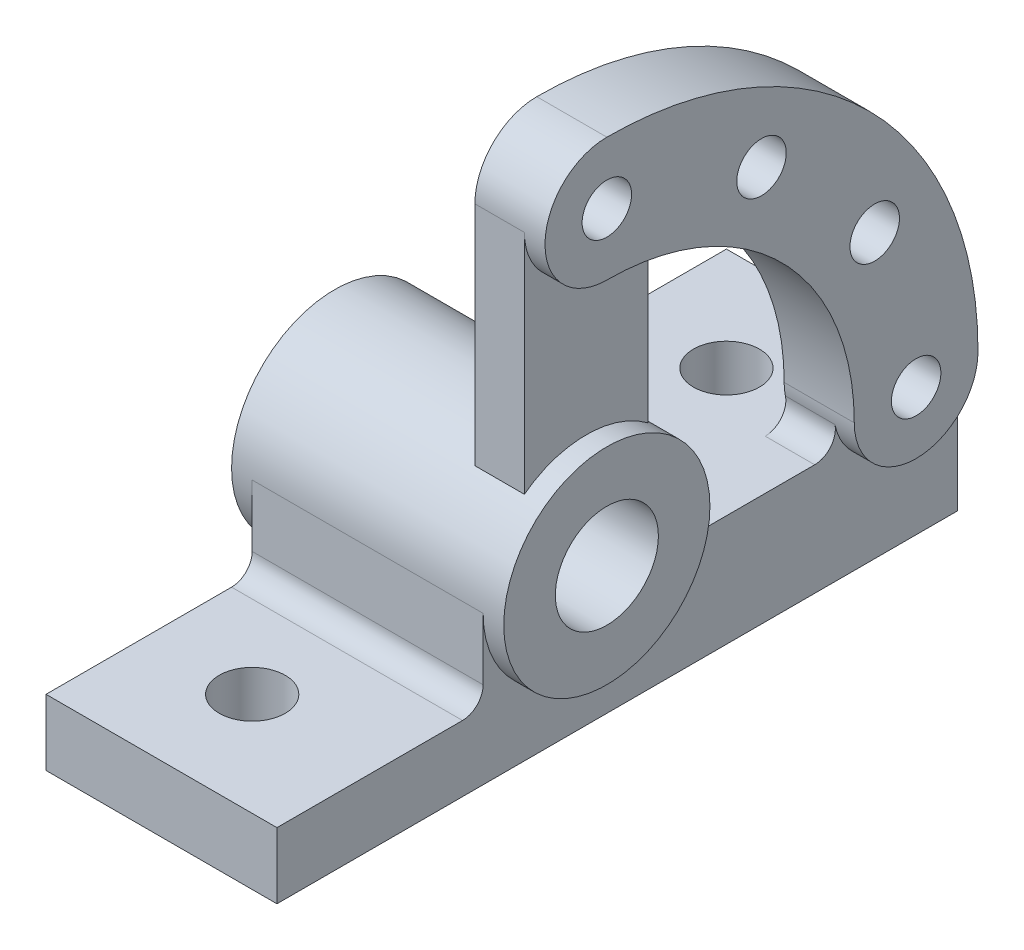
ISO-10303-21;
HEADER;
FILE_DESCRIPTION(('STEP AP214'),'2;1');
FILE_NAME('part.step','',(''),(''),'','','');
FILE_SCHEMA(('AUTOMOTIVE_DESIGN { 1 0 10303 214 1 1 1 1 }'));
ENDSEC;
DATA;
#1=APPLICATION_CONTEXT('core data for automotive mechanical design processes');
#2=APPLICATION_PROTOCOL_DEFINITION('international standard','automotive_design',2000,#1);
#3=PRODUCT_CONTEXT('',#1,'mechanical');
#4=PRODUCT('Part','Part','',(#3));
#5=PRODUCT_RELATED_PRODUCT_CATEGORY('part','',(#4));
#6=PRODUCT_DEFINITION_FORMATION('','',#4);
#7=PRODUCT_DEFINITION_CONTEXT('part definition',#1,'design');
#8=PRODUCT_DEFINITION('design','',#6,#7);
#9=PRODUCT_DEFINITION_SHAPE('','',#8);
#10=(LENGTH_UNIT() NAMED_UNIT(*) SI_UNIT(.MILLI.,.METRE.));
#11=(NAMED_UNIT(*) PLANE_ANGLE_UNIT() SI_UNIT($,.RADIAN.));
#12=(NAMED_UNIT(*) SI_UNIT($,.STERADIAN.) SOLID_ANGLE_UNIT());
#13=UNCERTAINTY_MEASURE_WITH_UNIT(LENGTH_MEASURE(1.E-05),#10,'distance_accuracy_value','');
#14=(GEOMETRIC_REPRESENTATION_CONTEXT(3) GLOBAL_UNCERTAINTY_ASSIGNED_CONTEXT((#13)) GLOBAL_UNIT_ASSIGNED_CONTEXT((#10,
#11,#12)) REPRESENTATION_CONTEXT('',''));
#15=CARTESIAN_POINT('',(0.,0.,0.));
#16=DIRECTION('',(0.,0.,1.));
#17=DIRECTION('',(1.,0.,0.));
#18=AXIS2_PLACEMENT_3D('',#15,#16,#17);
#19=CARTESIAN_POINT('',(16.,0.,0.));
#20=DIRECTION('',(1.,0.,0.));
#21=DIRECTION('',(0.,0.,-1.));
#22=AXIS2_PLACEMENT_3D('',#19,#20,#21);
#23=PLANE('',#22);
#24=CARTESIAN_POINT('',(16.,0.,-75.));
#25=DIRECTION('',(1.,0.,0.));
#26=DIRECTION('',(0.,0.,-1.));
#27=AXIS2_PLACEMENT_3D('',#24,#25,#26);
#28=CIRCLE('',#27,6.);
#29=CARTESIAN_POINT('',(16.,0.,-81.));
#30=VERTEX_POINT('',#29);
#31=EDGE_CURVE('E209',#30,#30,#28,.F.);
#32=ORIENTED_EDGE('',*,*,#31,.F.);
#33=EDGE_LOOP('',(#32));
#34=FACE_BOUND('',#33,.T.);
#35=CARTESIAN_POINT('',(16.,75.,2.61861100413235E-13));
#36=DIRECTION('',(1.,0.,0.));
#37=DIRECTION('',(0.,0.,-1.));
#38=AXIS2_PLACEMENT_3D('',#35,#36,#37);
#39=CIRCLE('',#38,6.);
#40=CARTESIAN_POINT('',(16.,75.,-5.99999999999974));
#41=VERTEX_POINT('',#40);
#42=EDGE_CURVE('E393',#41,#41,#39,.F.);
#43=ORIENTED_EDGE('',*,*,#42,.F.);
#44=EDGE_LOOP('',(#43));
#45=FACE_BOUND('',#44,.T.);
#46=CARTESIAN_POINT('',(16.,64.951905283833,-37.4999999999998));
#47=DIRECTION('',(1.,0.,0.));
#48=DIRECTION('',(0.,0.,-1.));
#49=AXIS2_PLACEMENT_3D('',#46,#47,#48);
#50=CIRCLE('',#49,6.);
#51=CARTESIAN_POINT('',(16.,64.951905283833,-43.4999999999999));
#52=VERTEX_POINT('',#51);
#53=EDGE_CURVE('E397',#52,#52,#50,.F.);
#54=ORIENTED_EDGE('',*,*,#53,.F.);
#55=EDGE_LOOP('',(#54));
#56=FACE_BOUND('',#55,.T.);
#57=CARTESIAN_POINT('',(16.,37.5000000000001,-64.9519052838328));
#58=DIRECTION('',(1.,0.,0.));
#59=DIRECTION('',(0.,0.,-1.));
#60=AXIS2_PLACEMENT_3D('',#57,#58,#59);
#61=CIRCLE('',#60,6.);
#62=CARTESIAN_POINT('',(16.,37.5000000000001,-70.9519052838329));
#63=VERTEX_POINT('',#62);
#64=EDGE_CURVE('E388',#63,#63,#61,.F.);
#65=ORIENTED_EDGE('',*,*,#64,.F.);
#66=EDGE_LOOP('',(#65));
#67=FACE_BOUND('',#66,.T.);
#68=CARTESIAN_POINT('',(16.,0.,0.));
#69=DIRECTION('',(1.,0.,0.));
#70=DIRECTION('',(0.,0.,-1.));
#71=AXIS2_PLACEMENT_3D('',#68,#69,#70);
#72=CIRCLE('',#71,90.);
#73=CARTESIAN_POINT('',(16.,90.,0.));
#74=VERTEX_POINT('',#73);
#75=CARTESIAN_POINT('',(16.,0.,-90.));
#76=VERTEX_POINT('',#75);
#77=EDGE_CURVE('E198',#74,#76,#72,.F.);
#78=ORIENTED_EDGE('',*,*,#77,.T.);
#79=DIRECTION('',(0.,1.,0.));
#80=VECTOR('',#79,1.);
#81=CARTESIAN_POINT('',(16.,0.,-90.));
#82=LINE('',#81,#80);
#83=CARTESIAN_POINT('',(16.,-9.,-90.));
#84=VERTEX_POINT('',#83);
#85=EDGE_CURVE('E12',#76,#84,#82,.F.);
#86=ORIENTED_EDGE('',*,*,#85,.T.);
#87=DIRECTION('',(0.,0.,-1.));
#88=VECTOR('',#87,1.);
#89=CARTESIAN_POINT('',(16.,-9.,0.));
#90=LINE('',#89,#88);
#91=CARTESIAN_POINT('',(16.,-9.,-55.4040820577346));
#92=VERTEX_POINT('',#91);
#93=EDGE_CURVE('E65',#92,#84,#90,.T.);
#94=ORIENTED_EDGE('',*,*,#93,.F.);
#95=CARTESIAN_POINT('',(16.,-4.,-55.4040820577346));
#96=DIRECTION('',(1.,0.,0.));
#97=DIRECTION('',(0.,0.,-1.));
#98=AXIS2_PLACEMENT_3D('',#95,#96,#97);
#99=CIRCLE('',#98,5.);
#100=CARTESIAN_POINT('',(16.,-3.,-60.3030615433009));
#101=VERTEX_POINT('',#100);
#102=EDGE_CURVE('E340',#92,#101,#99,.T.);
#103=ORIENTED_EDGE('',*,*,#102,.T.);
#104=CARTESIAN_POINT('',(16.,0.,-75.));
#105=DIRECTION('',(1.,0.,0.));
#106=DIRECTION('',(0.,0.,-1.));
#107=AXIS2_PLACEMENT_3D('',#104,#105,#106);
#108=CIRCLE('',#107,15.);
#109=CARTESIAN_POINT('',(16.,0.,-60.));
#110=VERTEX_POINT('',#109);
#111=EDGE_CURVE('E222',#101,#110,#108,.F.);
#112=ORIENTED_EDGE('',*,*,#111,.T.);
#113=CARTESIAN_POINT('',(16.,0.,0.));
#114=DIRECTION('',(1.,0.,0.));
#115=DIRECTION('',(0.,0.,-1.));
#116=AXIS2_PLACEMENT_3D('',#113,#114,#115);
#117=CIRCLE('',#116,60.);
#118=CARTESIAN_POINT('',(16.,58.0947501931113,-15.));
#119=VERTEX_POINT('',#118);
#120=EDGE_CURVE('E227',#119,#110,#117,.F.);
#121=ORIENTED_EDGE('',*,*,#120,.F.);
#122=DIRECTION('',(0.,1.,0.));
#123=VECTOR('',#122,1.);
#124=CARTESIAN_POINT('',(16.,0.,-15.));
#125=LINE('',#124,#123);
#126=CARTESIAN_POINT('',(16.,20.,-15.));
#127=VERTEX_POINT('',#126);
#128=EDGE_CURVE('E231',#127,#119,#125,.T.);
#129=ORIENTED_EDGE('',*,*,#128,.F.);
#130=CARTESIAN_POINT('',(16.,0.,0.));
#131=DIRECTION('',(1.,0.,0.));
#132=DIRECTION('',(0.,0.,-1.));
#133=AXIS2_PLACEMENT_3D('',#130,#131,#132);
#134=CIRCLE('',#133,25.);
#135=CARTESIAN_POINT('',(16.,20.,15.));
#136=VERTEX_POINT('',#135);
#137=EDGE_CURVE('E229',#127,#136,#134,.T.);
#138=ORIENTED_EDGE('',*,*,#137,.T.);
#139=DIRECTION('',(0.,1.,0.));
#140=VECTOR('',#139,1.);
#141=CARTESIAN_POINT('',(16.,0.,15.));
#142=LINE('',#141,#140);
#143=CARTESIAN_POINT('',(16.,75.,15.));
#144=VERTEX_POINT('',#143);
#145=EDGE_CURVE('E226',#136,#144,#142,.T.);
#146=ORIENTED_EDGE('',*,*,#145,.T.);
#147=CARTESIAN_POINT('',(16.,75.,0.));
#148=DIRECTION('',(1.,0.,0.));
#149=DIRECTION('',(0.,0.,-1.));
#150=AXIS2_PLACEMENT_3D('',#147,#148,#149);
#151=CIRCLE('',#150,15.);
#152=EDGE_CURVE('E369',#144,#74,#151,.F.);
#153=ORIENTED_EDGE('',*,*,#152,.T.);
#154=EDGE_LOOP('',(#78,#86,#94,#103,#112,#121,#129,#138,#146,#153));
#155=FACE_BOUND('',#154,.T.);
#156=ADVANCED_FACE('F50',(#34,#45,#56,#67,#155),#23,.F.);
#157=CARTESIAN_POINT('',(33.,0.,0.));
#158=DIRECTION('',(-1.,0.,0.));
#159=DIRECTION('',(0.,0.,1.));
#160=AXIS2_PLACEMENT_3D('',#157,#158,#159);
#161=CYLINDRICAL_SURFACE('',#160,25.);
#162=CARTESIAN_POINT('',(-33.,0.,0.));
#163=DIRECTION('',(1.,0.,0.));
#164=DIRECTION('',(0.,0.,-1.));
#165=AXIS2_PLACEMENT_3D('',#162,#163,#164);
#166=CIRCLE('',#165,25.);
#167=CARTESIAN_POINT('',(-33.,0.,-25.));
#168=VERTEX_POINT('',#167);
#169=EDGE_CURVE('E308',#168,#168,#166,.T.);
#170=ORIENTED_EDGE('',*,*,#169,.T.);
#171=EDGE_LOOP('',(#170));
#172=FACE_BOUND('',#171,.T.);
#173=CARTESIAN_POINT('',(33.,0.,0.));
#174=DIRECTION('',(1.,0.,0.));
#175=DIRECTION('',(0.,0.,-1.));
#176=AXIS2_PLACEMENT_3D('',#173,#174,#175);
#177=CIRCLE('',#176,25.);
#178=CARTESIAN_POINT('',(33.,0.,-25.));
#179=VERTEX_POINT('',#178);
#180=EDGE_CURVE('E311',#179,#179,#177,.T.);
#181=ORIENTED_EDGE('',*,*,#180,.F.);
#182=EDGE_LOOP('',(#181));
#183=FACE_BOUND('',#182,.T.);
#184=DIRECTION('',(-1.,0.,0.));
#185=VECTOR('',#184,1.);
#186=CARTESIAN_POINT('',(33.,-3.33333333333333,-24.7767812455308));
#187=LINE('',#186,#185);
#188=CARTESIAN_POINT('',(28.,-3.33333333333333,-24.7767812455308));
#189=VERTEX_POINT('',#188);
#190=CARTESIAN_POINT('',(-28.,-3.33333333333333,-24.7767812455308));
#191=VERTEX_POINT('',#190);
#192=EDGE_CURVE('E313',#189,#191,#187,.T.);
#193=ORIENTED_EDGE('',*,*,#192,.T.);
#194=CARTESIAN_POINT('',(-28.,0.,0.));
#195=DIRECTION('',(1.,0.,0.));
#196=DIRECTION('',(0.,0.,-1.));
#197=AXIS2_PLACEMENT_3D('',#194,#195,#196);
#198=CIRCLE('',#197,25.);
#199=CARTESIAN_POINT('',(-28.,0.,25.));
#200=VERTEX_POINT('',#199);
#201=EDGE_CURVE('E279',#200,#191,#198,.T.);
#202=ORIENTED_EDGE('',*,*,#201,.F.);
#203=DIRECTION('',(-1.,0.,0.));
#204=VECTOR('',#203,1.);
#205=CARTESIAN_POINT('',(28.,0.,25.));
#206=LINE('',#205,#204);
#207=CARTESIAN_POINT('',(28.,0.,25.));
#208=VERTEX_POINT('',#207);
#209=EDGE_CURVE('E301',#208,#200,#206,.T.);
#210=ORIENTED_EDGE('',*,*,#209,.F.);
#211=CARTESIAN_POINT('',(28.,0.,0.));
#212=DIRECTION('',(1.,0.,0.));
#213=DIRECTION('',(0.,0.,-1.));
#214=AXIS2_PLACEMENT_3D('',#211,#212,#213);
#215=CIRCLE('',#214,25.);
#216=EDGE_CURVE('E263',#208,#189,#215,.T.);
#217=ORIENTED_EDGE('',*,*,#216,.T.);
#218=EDGE_LOOP('',(#193,#202,#210,#217));
#219=FACE_BOUND('',#218,.T.);
#220=ORIENTED_EDGE('',*,*,#137,.F.);
#221=DIRECTION('',(1.,0.,0.));
#222=VECTOR('',#221,1.);
#223=CARTESIAN_POINT('',(16.,20.,-15.));
#224=LINE('',#223,#222);
#225=CARTESIAN_POINT('',(28.,20.,-15.));
#226=VERTEX_POINT('',#225);
#227=EDGE_CURVE('E250',#127,#226,#224,.T.);
#228=ORIENTED_EDGE('',*,*,#227,.T.);
#229=CARTESIAN_POINT('',(28.,0.,0.));
#230=DIRECTION('',(1.,0.,0.));
#231=DIRECTION('',(0.,0.,-1.));
#232=AXIS2_PLACEMENT_3D('',#229,#230,#231);
#233=CIRCLE('',#232,25.);
#234=CARTESIAN_POINT('',(28.,20.,15.));
#235=VERTEX_POINT('',#234);
#236=EDGE_CURVE('E239',#226,#235,#233,.T.);
#237=ORIENTED_EDGE('',*,*,#236,.T.);
#238=DIRECTION('',(1.,0.,0.));
#239=VECTOR('',#238,1.);
#240=CARTESIAN_POINT('',(16.,20.,15.));
#241=LINE('',#240,#239);
#242=EDGE_CURVE('E249',#136,#235,#241,.T.);
#243=ORIENTED_EDGE('',*,*,#242,.F.);
#244=EDGE_LOOP('',(#220,#228,#237,#243));
#245=FACE_BOUND('',#244,.T.);
#246=ADVANCED_FACE('F434',(#172,#183,#219,#245),#161,.T.);
#247=CARTESIAN_POINT('',(33.,0.,0.));
#248=DIRECTION('',(1.,0.,0.));
#249=DIRECTION('',(0.,0.,-1.));
#250=AXIS2_PLACEMENT_3D('',#247,#248,#249);
#251=PLANE('',#250);
#252=ORIENTED_EDGE('',*,*,#180,.T.);
#253=EDGE_LOOP('',(#252));
#254=FACE_BOUND('',#253,.T.);
#255=CARTESIAN_POINT('',(33.,0.,0.));
#256=DIRECTION('',(1.,0.,0.));
#257=DIRECTION('',(0.,0.,-1.));
#258=AXIS2_PLACEMENT_3D('',#255,#256,#257);
#259=CIRCLE('',#258,12.5);
#260=CARTESIAN_POINT('',(33.,0.,-12.5));
#261=VERTEX_POINT('',#260);
#262=EDGE_CURVE('E304',#261,#261,#259,.T.);
#263=ORIENTED_EDGE('',*,*,#262,.F.);
#264=EDGE_LOOP('',(#263));
#265=FACE_BOUND('',#264,.T.);
#266=ADVANCED_FACE('F442',(#254,#265),#251,.T.);
#267=CARTESIAN_POINT('',(-33.,0.,0.));
#268=DIRECTION('',(1.,0.,0.));
#269=DIRECTION('',(0.,0.,-1.));
#270=AXIS2_PLACEMENT_3D('',#267,#268,#269);
#271=PLANE('',#270);
#272=ORIENTED_EDGE('',*,*,#169,.F.);
#273=EDGE_LOOP('',(#272));
#274=FACE_BOUND('',#273,.T.);
#275=CARTESIAN_POINT('',(-33.,0.,0.));
#276=DIRECTION('',(1.,0.,0.));
#277=DIRECTION('',(0.,0.,-1.));
#278=AXIS2_PLACEMENT_3D('',#275,#276,#277);
#279=CIRCLE('',#278,12.5);
#280=CARTESIAN_POINT('',(-33.,0.,-12.5));
#281=VERTEX_POINT('',#280);
#282=EDGE_CURVE('E302',#281,#281,#279,.T.);
#283=ORIENTED_EDGE('',*,*,#282,.T.);
#284=EDGE_LOOP('',(#283));
#285=FACE_BOUND('',#284,.T.);
#286=ADVANCED_FACE('F490',(#274,#285),#271,.F.);
#287=CARTESIAN_POINT('',(33.,0.,0.));
#288=DIRECTION('',(-1.,0.,0.));
#289=DIRECTION('',(0.,0.,1.));
#290=AXIS2_PLACEMENT_3D('',#287,#288,#289);
#291=CYLINDRICAL_SURFACE('',#290,12.5);
#292=ORIENTED_EDGE('',*,*,#262,.T.);
#293=EDGE_LOOP('',(#292));
#294=FACE_BOUND('',#293,.T.);
#295=ORIENTED_EDGE('',*,*,#282,.F.);
#296=EDGE_LOOP('',(#295));
#297=FACE_BOUND('',#296,.T.);
#298=ADVANCED_FACE('F484',(#294,#297),#291,.F.);
#299=CARTESIAN_POINT('',(28.,-9.,0.));
#300=DIRECTION('',(0.,1.,0.));
#301=DIRECTION('',(0.,0.,1.));
#302=AXIS2_PLACEMENT_3D('',#299,#300,#301);
#303=PLANE('',#302);
#304=CARTESIAN_POINT('',(-3.,-9.,-65.));
#305=DIRECTION('',(0.,1.,0.));
#306=DIRECTION('',(0.,0.,1.));
#307=AXIS2_PLACEMENT_3D('',#304,#305,#306);
#308=CIRCLE('',#307,8.);
#309=CARTESIAN_POINT('',(-3.,-9.,-57.));
#310=VERTEX_POINT('',#309);
#311=EDGE_CURVE('E398',#310,#310,#308,.T.);
#312=ORIENTED_EDGE('',*,*,#311,.F.);
#313=EDGE_LOOP('',(#312));
#314=FACE_BOUND('',#313,.T.);
#315=DIRECTION('',(0.,0.,-1.));
#316=VECTOR('',#315,1.);
#317=CARTESIAN_POINT('',(-28.,-9.,0.));
#318=LINE('',#317,#316);
#319=CARTESIAN_POINT('',(-28.,-9.,-29.732137494637));
#320=VERTEX_POINT('',#319);
#321=CARTESIAN_POINT('',(-28.,-9.,-90.));
#322=VERTEX_POINT('',#321);
#323=EDGE_CURVE('E67',#320,#322,#318,.T.);
#324=ORIENTED_EDGE('',*,*,#323,.F.);
#325=DIRECTION('',(-1.,0.,0.));
#326=VECTOR('',#325,1.);
#327=CARTESIAN_POINT('',(28.,-9.,-29.732137494637));
#328=LINE('',#327,#326);
#329=CARTESIAN_POINT('',(28.,-9.,-29.732137494637));
#330=VERTEX_POINT('',#329);
#331=EDGE_CURVE('E325',#320,#330,#328,.F.);
#332=ORIENTED_EDGE('',*,*,#331,.T.);
#333=DIRECTION('',(0.,0.,-1.));
#334=VECTOR('',#333,1.);
#335=CARTESIAN_POINT('',(28.,-9.,0.));
#336=LINE('',#335,#334);
#337=CARTESIAN_POINT('',(28.,-9.,-55.4040820577346));
#338=VERTEX_POINT('',#337);
#339=EDGE_CURVE('E260',#330,#338,#336,.T.);
#340=ORIENTED_EDGE('',*,*,#339,.T.);
#341=DIRECTION('',(-1.,0.,0.));
#342=VECTOR('',#341,1.);
#343=CARTESIAN_POINT('',(16.,-9.,-55.4040820577346));
#344=LINE('',#343,#342);
#345=EDGE_CURVE('E318',#338,#92,#344,.T.);
#346=ORIENTED_EDGE('',*,*,#345,.T.);
#347=ORIENTED_EDGE('',*,*,#93,.T.);
#348=DIRECTION('',(1.,0.,0.));
#349=VECTOR('',#348,1.);
#350=CARTESIAN_POINT('',(28.,-9.,-90.));
#351=LINE('',#350,#349);
#352=EDGE_CURVE('E51',#322,#84,#351,.T.);
#353=ORIENTED_EDGE('',*,*,#352,.F.);
#354=EDGE_LOOP('',(#324,#332,#340,#346,#347,#353));
#355=FACE_BOUND('',#354,.T.);
#356=ADVANCED_FACE('F355',(#314,#355),#303,.T.);
#357=CARTESIAN_POINT('',(28.,0.,25.));
#358=DIRECTION('',(0.,0.,1.));
#359=DIRECTION('',(1.,0.,0.));
#360=AXIS2_PLACEMENT_3D('',#357,#358,#359);
#361=PLANE('',#360);
#362=DIRECTION('',(0.,1.,0.));
#363=VECTOR('',#362,1.);
#364=CARTESIAN_POINT('',(-28.,0.,25.));
#365=LINE('',#364,#363);
#366=CARTESIAN_POINT('',(-28.,-15.,25.));
#367=VERTEX_POINT('',#366);
#368=EDGE_CURVE('E278',#367,#200,#365,.T.);
#369=ORIENTED_EDGE('',*,*,#368,.F.);
#370=DIRECTION('',(-1.,0.,0.));
#371=VECTOR('',#370,1.);
#372=CARTESIAN_POINT('',(28.,-15.,25.));
#373=LINE('',#372,#371);
#374=CARTESIAN_POINT('',(28.,-15.,25.));
#375=VERTEX_POINT('',#374);
#376=EDGE_CURVE('E329',#367,#375,#373,.F.);
#377=ORIENTED_EDGE('',*,*,#376,.T.);
#378=DIRECTION('',(0.,1.,0.));
#379=VECTOR('',#378,1.);
#380=CARTESIAN_POINT('',(28.,0.,25.));
#381=LINE('',#380,#379);
#382=EDGE_CURVE('E261',#375,#208,#381,.T.);
#383=ORIENTED_EDGE('',*,*,#382,.T.);
#384=ORIENTED_EDGE('',*,*,#209,.T.);
#385=EDGE_LOOP('',(#369,#377,#383,#384));
#386=FACE_BOUND('',#385,.T.);
#387=ADVANCED_FACE('F476',(#386),#361,.T.);
#388=CARTESIAN_POINT('',(28.,-20.,0.));
#389=DIRECTION('',(0.,1.,0.));
#390=DIRECTION('',(0.,0.,1.));
#391=AXIS2_PLACEMENT_3D('',#388,#389,#390);
#392=PLANE('',#391);
#393=CARTESIAN_POINT('',(-3.,-20.,50.));
#394=DIRECTION('',(0.,1.,0.));
#395=DIRECTION('',(0.,0.,1.));
#396=AXIS2_PLACEMENT_3D('',#393,#394,#395);
#397=CIRCLE('',#396,8.);
#398=CARTESIAN_POINT('',(-3.,-20.,58.));
#399=VERTEX_POINT('',#398);
#400=EDGE_CURVE('E413',#399,#399,#397,.T.);
#401=ORIENTED_EDGE('',*,*,#400,.F.);
#402=EDGE_LOOP('',(#401));
#403=FACE_BOUND('',#402,.T.);
#404=DIRECTION('',(0.,0.,-1.));
#405=VECTOR('',#404,1.);
#406=CARTESIAN_POINT('',(28.,-20.,0.));
#407=LINE('',#406,#405);
#408=CARTESIAN_POINT('',(28.,-20.,75.));
#409=VERTEX_POINT('',#408);
#410=CARTESIAN_POINT('',(28.,-20.,30.));
#411=VERTEX_POINT('',#410);
#412=EDGE_CURVE('E264',#409,#411,#407,.T.);
#413=ORIENTED_EDGE('',*,*,#412,.T.);
#414=DIRECTION('',(-1.,0.,0.));
#415=VECTOR('',#414,1.);
#416=CARTESIAN_POINT('',(-28.,-20.,30.));
#417=LINE('',#416,#415);
#418=CARTESIAN_POINT('',(-28.,-20.,30.));
#419=VERTEX_POINT('',#418);
#420=EDGE_CURVE('E330',#411,#419,#417,.T.);
#421=ORIENTED_EDGE('',*,*,#420,.T.);
#422=DIRECTION('',(0.,0.,-1.));
#423=VECTOR('',#422,1.);
#424=CARTESIAN_POINT('',(-28.,-20.,0.));
#425=LINE('',#424,#423);
#426=CARTESIAN_POINT('',(-28.,-20.,75.));
#427=VERTEX_POINT('',#426);
#428=EDGE_CURVE('E285',#427,#419,#425,.T.);
#429=ORIENTED_EDGE('',*,*,#428,.F.);
#430=DIRECTION('',(-1.,0.,0.));
#431=VECTOR('',#430,1.);
#432=CARTESIAN_POINT('',(28.,-20.,75.));
#433=LINE('',#432,#431);
#434=EDGE_CURVE('E299',#409,#427,#433,.T.);
#435=ORIENTED_EDGE('',*,*,#434,.F.);
#436=EDGE_LOOP('',(#413,#421,#429,#435));
#437=FACE_BOUND('',#436,.T.);
#438=ADVANCED_FACE('F471',(#403,#437),#392,.T.);
#439=CARTESIAN_POINT('',(28.,0.,75.));
#440=DIRECTION('',(0.,0.,1.));
#441=DIRECTION('',(1.,0.,0.));
#442=AXIS2_PLACEMENT_3D('',#439,#440,#441);
#443=PLANE('',#442);
#444=DIRECTION('',(0.,1.,0.));
#445=VECTOR('',#444,1.);
#446=CARTESIAN_POINT('',(-28.,0.,75.));
#447=LINE('',#446,#445);
#448=CARTESIAN_POINT('',(-28.,-36.,75.));
#449=VERTEX_POINT('',#448);
#450=EDGE_CURVE('E284',#449,#427,#447,.T.);
#451=ORIENTED_EDGE('',*,*,#450,.F.);
#452=DIRECTION('',(-1.,0.,0.));
#453=VECTOR('',#452,1.);
#454=CARTESIAN_POINT('',(28.,-36.,75.));
#455=LINE('',#454,#453);
#456=CARTESIAN_POINT('',(28.,-36.,75.));
#457=VERTEX_POINT('',#456);
#458=EDGE_CURVE('E300',#457,#449,#455,.T.);
#459=ORIENTED_EDGE('',*,*,#458,.F.);
#460=DIRECTION('',(0.,1.,0.));
#461=VECTOR('',#460,1.);
#462=CARTESIAN_POINT('',(28.,0.,75.));
#463=LINE('',#462,#461);
#464=EDGE_CURVE('E268',#457,#409,#463,.T.);
#465=ORIENTED_EDGE('',*,*,#464,.T.);
#466=ORIENTED_EDGE('',*,*,#434,.T.);
#467=EDGE_LOOP('',(#451,#459,#465,#466));
#468=FACE_BOUND('',#467,.T.);
#469=ADVANCED_FACE('F472',(#468),#443,.T.);
#470=CARTESIAN_POINT('',(28.,-36.,0.));
#471=DIRECTION('',(0.,1.,0.));
#472=DIRECTION('',(0.,0.,1.));
#473=AXIS2_PLACEMENT_3D('',#470,#471,#472);
#474=PLANE('',#473);
#475=CARTESIAN_POINT('',(-3.,-36.,-65.));
#476=DIRECTION('',(0.,1.,0.));
#477=DIRECTION('',(0.,0.,1.));
#478=AXIS2_PLACEMENT_3D('',#475,#476,#477);
#479=CIRCLE('',#478,8.);
#480=CARTESIAN_POINT('',(-3.,-36.,-57.));
#481=VERTEX_POINT('',#480);
#482=EDGE_CURVE('E412',#481,#481,#479,.T.);
#483=ORIENTED_EDGE('',*,*,#482,.T.);
#484=EDGE_LOOP('',(#483));
#485=FACE_BOUND('',#484,.T.);
#486=CARTESIAN_POINT('',(-3.,-36.,50.));
#487=DIRECTION('',(0.,1.,0.));
#488=DIRECTION('',(0.,0.,1.));
#489=AXIS2_PLACEMENT_3D('',#486,#487,#488);
#490=CIRCLE('',#489,8.);
#491=CARTESIAN_POINT('',(-3.,-36.,58.));
#492=VERTEX_POINT('',#491);
#493=EDGE_CURVE('E414',#492,#492,#490,.T.);
#494=ORIENTED_EDGE('',*,*,#493,.T.);
#495=EDGE_LOOP('',(#494));
#496=FACE_BOUND('',#495,.T.);
#497=DIRECTION('',(0.,0.,-1.));
#498=VECTOR('',#497,1.);
#499=CARTESIAN_POINT('',(-28.,-36.,0.));
#500=LINE('',#499,#498);
#501=CARTESIAN_POINT('',(-28.,-36.,-90.));
#502=VERTEX_POINT('',#501);
#503=EDGE_CURVE('E288',#449,#502,#500,.T.);
#504=ORIENTED_EDGE('',*,*,#503,.T.);
#505=DIRECTION('',(-1.,0.,0.));
#506=VECTOR('',#505,1.);
#507=CARTESIAN_POINT('',(28.,-36.,-90.));
#508=LINE('',#507,#506);
#509=CARTESIAN_POINT('',(28.,-36.,-90.));
#510=VERTEX_POINT('',#509);
#511=EDGE_CURVE('E295',#510,#502,#508,.T.);
#512=ORIENTED_EDGE('',*,*,#511,.F.);
#513=DIRECTION('',(0.,0.,-1.));
#514=VECTOR('',#513,1.);
#515=CARTESIAN_POINT('',(28.,-36.,0.));
#516=LINE('',#515,#514);
#517=EDGE_CURVE('E272',#457,#510,#516,.T.);
#518=ORIENTED_EDGE('',*,*,#517,.F.);
#519=ORIENTED_EDGE('',*,*,#458,.T.);
#520=EDGE_LOOP('',(#504,#512,#518,#519));
#521=FACE_BOUND('',#520,.T.);
#522=ADVANCED_FACE('F423',(#485,#496,#521),#474,.F.);
#523=CARTESIAN_POINT('',(28.,0.,-90.));
#524=DIRECTION('',(0.,0.,1.));
#525=DIRECTION('',(1.,0.,0.));
#526=AXIS2_PLACEMENT_3D('',#523,#524,#525);
#527=PLANE('',#526);
#528=DIRECTION('',(0.,1.,0.));
#529=VECTOR('',#528,1.);
#530=CARTESIAN_POINT('',(-28.,0.,-90.));
#531=LINE('',#530,#529);
#532=EDGE_CURVE('E259',#502,#322,#531,.T.);
#533=ORIENTED_EDGE('',*,*,#532,.T.);
#534=ORIENTED_EDGE('',*,*,#352,.T.);
#535=ORIENTED_EDGE('',*,*,#85,.F.);
#536=DIRECTION('',(-1.,0.,0.));
#537=VECTOR('',#536,1.);
#538=CARTESIAN_POINT('',(28.,0.,-90.));
#539=LINE('',#538,#537);
#540=CARTESIAN_POINT('',(28.,0.,-90.));
#541=VERTEX_POINT('',#540);
#542=EDGE_CURVE('E277',#541,#76,#539,.T.);
#543=ORIENTED_EDGE('',*,*,#542,.F.);
#544=DIRECTION('',(0.,1.,0.));
#545=VECTOR('',#544,1.);
#546=CARTESIAN_POINT('',(28.,0.,-90.));
#547=LINE('',#546,#545);
#548=EDGE_CURVE('E271',#510,#541,#547,.T.);
#549=ORIENTED_EDGE('',*,*,#548,.F.);
#550=ORIENTED_EDGE('',*,*,#511,.T.);
#551=EDGE_LOOP('',(#533,#534,#535,#543,#549,#550));
#552=FACE_BOUND('',#551,.T.);
#553=ADVANCED_FACE('F349',(#552),#527,.F.);
#554=CARTESIAN_POINT('',(28.,0.,0.));
#555=DIRECTION('',(1.,0.,0.));
#556=DIRECTION('',(0.,0.,-1.));
#557=AXIS2_PLACEMENT_3D('',#554,#555,#556);
#558=PLANE('',#557);
#559=CARTESIAN_POINT('',(28.,0.,-75.));
#560=DIRECTION('',(1.,0.,0.));
#561=DIRECTION('',(0.,0.,-1.));
#562=AXIS2_PLACEMENT_3D('',#559,#560,#561);
#563=CIRCLE('',#562,15.);
#564=CARTESIAN_POINT('',(28.,-3.,-60.3030615433009));
#565=VERTEX_POINT('',#564);
#566=EDGE_CURVE('E251',#565,#541,#563,.T.);
#567=ORIENTED_EDGE('',*,*,#566,.F.);
#568=CARTESIAN_POINT('',(28.,-4.,-55.4040820577346));
#569=DIRECTION('',(1.,0.,0.));
#570=DIRECTION('',(0.,0.,-1.));
#571=AXIS2_PLACEMENT_3D('',#568,#569,#570);
#572=CIRCLE('',#571,5.);
#573=EDGE_CURVE('E339',#565,#338,#572,.F.);
#574=ORIENTED_EDGE('',*,*,#573,.T.);
#575=ORIENTED_EDGE('',*,*,#339,.F.);
#576=CARTESIAN_POINT('',(28.,-4.,-29.732137494637));
#577=DIRECTION('',(1.,0.,0.));
#578=DIRECTION('',(0.,0.,-1.));
#579=AXIS2_PLACEMENT_3D('',#576,#577,#578);
#580=CIRCLE('',#579,5.);
#581=EDGE_CURVE('E332',#330,#189,#580,.F.);
#582=ORIENTED_EDGE('',*,*,#581,.T.);
#583=ORIENTED_EDGE('',*,*,#216,.F.);
#584=ORIENTED_EDGE('',*,*,#382,.F.);
#585=CARTESIAN_POINT('',(28.,-15.,30.));
#586=DIRECTION('',(1.,0.,0.));
#587=DIRECTION('',(0.,0.,-1.));
#588=AXIS2_PLACEMENT_3D('',#585,#586,#587);
#589=CIRCLE('',#588,5.);
#590=EDGE_CURVE('E344',#375,#411,#589,.F.);
#591=ORIENTED_EDGE('',*,*,#590,.T.);
#592=ORIENTED_EDGE('',*,*,#412,.F.);
#593=ORIENTED_EDGE('',*,*,#464,.F.);
#594=ORIENTED_EDGE('',*,*,#517,.T.);
#595=ORIENTED_EDGE('',*,*,#548,.T.);
#596=EDGE_LOOP('',(#567,#574,#575,#582,#583,#584,#591,#592,#593,#594,#595));
#597=FACE_BOUND('',#596,.T.);
#598=ADVANCED_FACE('F363',(#597),#558,.T.);
#599=CARTESIAN_POINT('',(-28.,0.,0.));
#600=DIRECTION('',(1.,0.,0.));
#601=DIRECTION('',(0.,0.,-1.));
#602=AXIS2_PLACEMENT_3D('',#599,#600,#601);
#603=PLANE('',#602);
#604=ORIENTED_EDGE('',*,*,#323,.T.);
#605=ORIENTED_EDGE('',*,*,#532,.F.);
#606=ORIENTED_EDGE('',*,*,#503,.F.);
#607=ORIENTED_EDGE('',*,*,#450,.T.);
#608=ORIENTED_EDGE('',*,*,#428,.T.);
#609=CARTESIAN_POINT('',(-28.,-15.,30.));
#610=DIRECTION('',(1.,0.,0.));
#611=DIRECTION('',(0.,0.,-1.));
#612=AXIS2_PLACEMENT_3D('',#609,#610,#611);
#613=CIRCLE('',#612,5.);
#614=EDGE_CURVE('E342',#419,#367,#613,.T.);
#615=ORIENTED_EDGE('',*,*,#614,.T.);
#616=ORIENTED_EDGE('',*,*,#368,.T.);
#617=ORIENTED_EDGE('',*,*,#201,.T.);
#618=CARTESIAN_POINT('',(-28.,-4.,-29.732137494637));
#619=DIRECTION('',(1.,0.,0.));
#620=DIRECTION('',(0.,0.,-1.));
#621=AXIS2_PLACEMENT_3D('',#618,#619,#620);
#622=CIRCLE('',#621,5.);
#623=EDGE_CURVE('E335',#191,#320,#622,.T.);
#624=ORIENTED_EDGE('',*,*,#623,.T.);
#625=EDGE_LOOP('',(#604,#605,#606,#607,#608,#615,#616,#617,#624));
#626=FACE_BOUND('',#625,.T.);
#627=ADVANCED_FACE('F457',(#626),#603,.F.);
#628=CARTESIAN_POINT('',(16.,0.,-15.));
#629=DIRECTION('',(0.,0.,-1.));
#630=DIRECTION('',(0.,1.,0.));
#631=AXIS2_PLACEMENT_3D('',#628,#629,#630);
#632=PLANE('',#631);
#633=DIRECTION('',(0.,1.,0.));
#634=VECTOR('',#633,1.);
#635=CARTESIAN_POINT('',(28.,0.,-15.));
#636=LINE('',#635,#634);
#637=CARTESIAN_POINT('',(28.,58.0947501931113,-15.));
#638=VERTEX_POINT('',#637);
#639=EDGE_CURVE('E233',#226,#638,#636,.T.);
#640=ORIENTED_EDGE('',*,*,#639,.F.);
#641=ORIENTED_EDGE('',*,*,#227,.F.);
#642=ORIENTED_EDGE('',*,*,#128,.T.);
#643=DIRECTION('',(1.,0.,0.));
#644=VECTOR('',#643,1.);
#645=CARTESIAN_POINT('',(16.,58.0947501931113,-15.));
#646=LINE('',#645,#644);
#647=EDGE_CURVE('E244',#119,#638,#646,.T.);
#648=ORIENTED_EDGE('',*,*,#647,.T.);
#649=EDGE_LOOP('',(#640,#641,#642,#648));
#650=FACE_BOUND('',#649,.T.);
#651=ADVANCED_FACE('F458',(#650),#632,.T.);
#652=CARTESIAN_POINT('',(16.,0.,15.));
#653=DIRECTION('',(0.,0.,-1.));
#654=DIRECTION('',(0.,1.,0.));
#655=AXIS2_PLACEMENT_3D('',#652,#653,#654);
#656=PLANE('',#655);
#657=DIRECTION('',(0.,1.,0.));
#658=VECTOR('',#657,1.);
#659=CARTESIAN_POINT('',(28.,0.,15.));
#660=LINE('',#659,#658);
#661=CARTESIAN_POINT('',(28.,75.,15.));
#662=VERTEX_POINT('',#661);
#663=EDGE_CURVE('E238',#235,#662,#660,.T.);
#664=ORIENTED_EDGE('',*,*,#663,.T.);
#665=DIRECTION('',(1.,0.,0.));
#666=VECTOR('',#665,1.);
#667=CARTESIAN_POINT('',(16.,75.,15.));
#668=LINE('',#667,#666);
#669=EDGE_CURVE('E232',#144,#662,#668,.T.);
#670=ORIENTED_EDGE('',*,*,#669,.F.);
#671=ORIENTED_EDGE('',*,*,#145,.F.);
#672=ORIENTED_EDGE('',*,*,#242,.T.);
#673=EDGE_LOOP('',(#664,#670,#671,#672));
#674=FACE_BOUND('',#673,.T.);
#675=ADVANCED_FACE('F451',(#674),#656,.F.);
#676=CARTESIAN_POINT('',(28.,0.,0.));
#677=DIRECTION('',(1.,0.,0.));
#678=DIRECTION('',(0.,0.,-1.));
#679=AXIS2_PLACEMENT_3D('',#676,#677,#678);
#680=PLANE('',#679);
#681=CARTESIAN_POINT('',(28.,0.,0.));
#682=DIRECTION('',(1.,0.,0.));
#683=DIRECTION('',(0.,0.,-1.));
#684=AXIS2_PLACEMENT_3D('',#681,#682,#683);
#685=CIRCLE('',#684,60.);
#686=CARTESIAN_POINT('',(28.,60.,0.));
#687=VERTEX_POINT('',#686);
#688=EDGE_CURVE('E228',#638,#687,#685,.T.);
#689=ORIENTED_EDGE('',*,*,#688,.T.);
#690=CARTESIAN_POINT('',(28.,75.,0.));
#691=DIRECTION('',(1.,0.,0.));
#692=DIRECTION('',(0.,0.,-1.));
#693=AXIS2_PLACEMENT_3D('',#690,#691,#692);
#694=CIRCLE('',#693,15.);
#695=EDGE_CURVE('E194',#662,#687,#694,.T.);
#696=ORIENTED_EDGE('',*,*,#695,.F.);
#697=ORIENTED_EDGE('',*,*,#663,.F.);
#698=ORIENTED_EDGE('',*,*,#236,.F.);
#699=ORIENTED_EDGE('',*,*,#639,.T.);
#700=EDGE_LOOP('',(#689,#696,#697,#698,#699));
#701=FACE_BOUND('',#700,.T.);
#702=ADVANCED_FACE('F452',(#701),#680,.T.);
#703=CARTESIAN_POINT('',(-132.492424049175,0.,-75.));
#704=DIRECTION('',(1.,0.,0.));
#705=DIRECTION('',(0.,0.,-1.));
#706=AXIS2_PLACEMENT_3D('',#703,#704,#705);
#707=CYLINDRICAL_SURFACE('',#706,15.);
#708=ORIENTED_EDGE('',*,*,#111,.F.);
#709=DIRECTION('',(1.,0.,0.));
#710=VECTOR('',#709,1.);
#711=CARTESIAN_POINT('',(-132.492424049175,-3.,-60.3030615433009));
#712=LINE('',#711,#710);
#713=EDGE_CURVE('E321',#101,#565,#712,.T.);
#714=ORIENTED_EDGE('',*,*,#713,.T.);
#715=ORIENTED_EDGE('',*,*,#566,.T.);
#716=DIRECTION('',(1.,0.,0.));
#717=VECTOR('',#716,1.);
#718=CARTESIAN_POINT('',(-132.492424049175,0.,-90.));
#719=LINE('',#718,#717);
#720=CARTESIAN_POINT('',(33.,0.,-90.));
#721=VERTEX_POINT('',#720);
#722=EDGE_CURVE('E221',#541,#721,#719,.T.);
#723=ORIENTED_EDGE('',*,*,#722,.T.);
#724=CARTESIAN_POINT('',(33.,0.,-75.));
#725=DIRECTION('',(1.,0.,0.));
#726=DIRECTION('',(0.,0.,-1.));
#727=AXIS2_PLACEMENT_3D('',#724,#725,#726);
#728=CIRCLE('',#727,15.);
#729=CARTESIAN_POINT('',(33.,0.,-60.));
#730=VERTEX_POINT('',#729);
#731=EDGE_CURVE('E213',#730,#721,#728,.T.);
#732=ORIENTED_EDGE('',*,*,#731,.F.);
#733=DIRECTION('',(1.,0.,0.));
#734=VECTOR('',#733,1.);
#735=CARTESIAN_POINT('',(-132.492424049175,0.,-60.));
#736=LINE('',#735,#734);
#737=EDGE_CURVE('E204',#110,#730,#736,.T.);
#738=ORIENTED_EDGE('',*,*,#737,.F.);
#739=EDGE_LOOP('',(#708,#714,#715,#723,#732,#738));
#740=FACE_BOUND('',#739,.T.);
#741=ADVANCED_FACE('F379',(#740),#707,.T.);
#742=CARTESIAN_POINT('',(-132.492424049175,0.,0.));
#743=DIRECTION('',(1.,0.,0.));
#744=DIRECTION('',(0.,0.,-1.));
#745=AXIS2_PLACEMENT_3D('',#742,#743,#744);
#746=CYLINDRICAL_SURFACE('',#745,60.);
#747=ORIENTED_EDGE('',*,*,#647,.F.);
#748=ORIENTED_EDGE('',*,*,#120,.T.);
#749=ORIENTED_EDGE('',*,*,#737,.T.);
#750=CARTESIAN_POINT('',(33.,0.,0.));
#751=DIRECTION('',(1.,0.,0.));
#752=DIRECTION('',(0.,0.,-1.));
#753=AXIS2_PLACEMENT_3D('',#750,#751,#752);
#754=CIRCLE('',#753,60.);
#755=CARTESIAN_POINT('',(33.,60.,0.));
#756=VERTEX_POINT('',#755);
#757=EDGE_CURVE('E199',#730,#756,#754,.T.);
#758=ORIENTED_EDGE('',*,*,#757,.T.);
#759=DIRECTION('',(1.,0.,0.));
#760=VECTOR('',#759,1.);
#761=CARTESIAN_POINT('',(-132.492424049175,60.,0.));
#762=LINE('',#761,#760);
#763=EDGE_CURVE('E182',#687,#756,#762,.T.);
#764=ORIENTED_EDGE('',*,*,#763,.F.);
#765=ORIENTED_EDGE('',*,*,#688,.F.);
#766=EDGE_LOOP('',(#747,#748,#749,#758,#764,#765));
#767=FACE_BOUND('',#766,.T.);
#768=ADVANCED_FACE('F205',(#767),#746,.F.);
#769=CARTESIAN_POINT('',(-132.492424049175,75.,0.));
#770=DIRECTION('',(1.,0.,0.));
#771=DIRECTION('',(0.,0.,-1.));
#772=AXIS2_PLACEMENT_3D('',#769,#770,#771);
#773=CYLINDRICAL_SURFACE('',#772,15.);
#774=ORIENTED_EDGE('',*,*,#152,.F.);
#775=ORIENTED_EDGE('',*,*,#669,.T.);
#776=ORIENTED_EDGE('',*,*,#695,.T.);
#777=ORIENTED_EDGE('',*,*,#763,.T.);
#778=CARTESIAN_POINT('',(33.,75.,0.));
#779=DIRECTION('',(1.,0.,0.));
#780=DIRECTION('',(0.,0.,-1.));
#781=AXIS2_PLACEMENT_3D('',#778,#779,#780);
#782=CIRCLE('',#781,15.);
#783=CARTESIAN_POINT('',(33.,90.,0.));
#784=VERTEX_POINT('',#783);
#785=EDGE_CURVE('E186',#784,#756,#782,.T.);
#786=ORIENTED_EDGE('',*,*,#785,.F.);
#787=DIRECTION('',(1.,0.,0.));
#788=VECTOR('',#787,1.);
#789=CARTESIAN_POINT('',(-132.492424049175,90.,0.));
#790=LINE('',#789,#788);
#791=EDGE_CURVE('E200',#74,#784,#790,.T.);
#792=ORIENTED_EDGE('',*,*,#791,.F.);
#793=EDGE_LOOP('',(#774,#775,#776,#777,#786,#792));
#794=FACE_BOUND('',#793,.T.);
#795=ADVANCED_FACE('F187',(#794),#773,.T.);
#796=CARTESIAN_POINT('',(-132.492424049175,0.,0.));
#797=DIRECTION('',(1.,0.,0.));
#798=DIRECTION('',(0.,0.,-1.));
#799=AXIS2_PLACEMENT_3D('',#796,#797,#798);
#800=CYLINDRICAL_SURFACE('',#799,90.);
#801=ORIENTED_EDGE('',*,*,#77,.F.);
#802=ORIENTED_EDGE('',*,*,#791,.T.);
#803=CARTESIAN_POINT('',(33.,0.,0.));
#804=DIRECTION('',(1.,0.,0.));
#805=DIRECTION('',(0.,0.,-1.));
#806=AXIS2_PLACEMENT_3D('',#803,#804,#805);
#807=CIRCLE('',#806,90.);
#808=EDGE_CURVE('E214',#721,#784,#807,.T.);
#809=ORIENTED_EDGE('',*,*,#808,.F.);
#810=ORIENTED_EDGE('',*,*,#722,.F.);
#811=ORIENTED_EDGE('',*,*,#542,.T.);
#812=EDGE_LOOP('',(#801,#802,#809,#810,#811));
#813=FACE_BOUND('',#812,.T.);
#814=ADVANCED_FACE('F372',(#813),#800,.T.);
#815=CARTESIAN_POINT('',(33.,37.5,0.));
#816=DIRECTION('',(1.,0.,0.));
#817=DIRECTION('',(0.,0.,-1.));
#818=AXIS2_PLACEMENT_3D('',#815,#816,#817);
#819=PLANE('',#818);
#820=CARTESIAN_POINT('',(33.,37.5000000000001,-64.9519052838328));
#821=DIRECTION('',(1.,0.,0.));
#822=DIRECTION('',(0.,0.500000000000001,-0.866025403784438));
#823=AXIS2_PLACEMENT_3D('',#820,#821,#822);
#824=CIRCLE('',#823,6.);
#825=CARTESIAN_POINT('',(33.,40.5000000000001,-70.1480577065395));
#826=VERTEX_POINT('',#825);
#827=EDGE_CURVE('E405',#826,#826,#824,.T.);
#828=ORIENTED_EDGE('',*,*,#827,.F.);
#829=EDGE_LOOP('',(#828));
#830=FACE_BOUND('',#829,.T.);
#831=CARTESIAN_POINT('',(33.,64.951905283833,-37.4999999999998));
#832=DIRECTION('',(1.,0.,0.));
#833=DIRECTION('',(0.,0.86602540378444,-0.499999999999998));
#834=AXIS2_PLACEMENT_3D('',#831,#832,#833);
#835=CIRCLE('',#834,6.);
#836=CARTESIAN_POINT('',(33.,70.1480577065396,-40.4999999999998));
#837=VERTEX_POINT('',#836);
#838=EDGE_CURVE('E392',#837,#837,#835,.T.);
#839=ORIENTED_EDGE('',*,*,#838,.F.);
#840=EDGE_LOOP('',(#839));
#841=FACE_BOUND('',#840,.T.);
#842=CARTESIAN_POINT('',(33.,75.,2.61861100413235E-13));
#843=DIRECTION('',(1.,0.,0.));
#844=DIRECTION('',(0.,1.,0.));
#845=AXIS2_PLACEMENT_3D('',#842,#843,#844);
#846=CIRCLE('',#845,6.);
#847=CARTESIAN_POINT('',(33.,81.,2.82809988446294E-13));
#848=VERTEX_POINT('',#847);
#849=EDGE_CURVE('E394',#848,#848,#846,.T.);
#850=ORIENTED_EDGE('',*,*,#849,.F.);
#851=EDGE_LOOP('',(#850));
#852=FACE_BOUND('',#851,.T.);
#853=CARTESIAN_POINT('',(33.,0.,-75.));
#854=DIRECTION('',(1.,0.,0.));
#855=DIRECTION('',(0.,0.,-1.));
#856=AXIS2_PLACEMENT_3D('',#853,#854,#855);
#857=CIRCLE('',#856,6.);
#858=CARTESIAN_POINT('',(33.,0.,-81.));
#859=VERTEX_POINT('',#858);
#860=EDGE_CURVE('E390',#859,#859,#857,.T.);
#861=ORIENTED_EDGE('',*,*,#860,.F.);
#862=EDGE_LOOP('',(#861));
#863=FACE_BOUND('',#862,.T.);
#864=ORIENTED_EDGE('',*,*,#757,.F.);
#865=ORIENTED_EDGE('',*,*,#731,.T.);
#866=ORIENTED_EDGE('',*,*,#808,.T.);
#867=ORIENTED_EDGE('',*,*,#785,.T.);
#868=EDGE_LOOP('',(#864,#865,#866,#867));
#869=FACE_BOUND('',#868,.T.);
#870=ADVANCED_FACE('F212',(#830,#841,#852,#863,#869),#819,.T.);
#871=CARTESIAN_POINT('',(-33.001,0.,-75.));
#872=DIRECTION('',(1.,0.,0.));
#873=DIRECTION('',(0.,0.,-1.));
#874=AXIS2_PLACEMENT_3D('',#871,#872,#873);
#875=CYLINDRICAL_SURFACE('',#874,6.);
#876=ORIENTED_EDGE('',*,*,#860,.T.);
#877=EDGE_LOOP('',(#876));
#878=FACE_BOUND('',#877,.T.);
#879=ORIENTED_EDGE('',*,*,#31,.T.);
#880=EDGE_LOOP('',(#879));
#881=FACE_BOUND('',#880,.T.);
#882=ADVANCED_FACE('F626',(#878,#881),#875,.F.);
#883=CARTESIAN_POINT('',(-33.001,75.,2.61861100413235E-13));
#884=DIRECTION('',(1.,0.,0.));
#885=DIRECTION('',(0.,0.,-1.));
#886=AXIS2_PLACEMENT_3D('',#883,#884,#885);
#887=CYLINDRICAL_SURFACE('',#886,6.);
#888=ORIENTED_EDGE('',*,*,#849,.T.);
#889=EDGE_LOOP('',(#888));
#890=FACE_BOUND('',#889,.T.);
#891=ORIENTED_EDGE('',*,*,#42,.T.);
#892=EDGE_LOOP('',(#891));
#893=FACE_BOUND('',#892,.T.);
#894=ADVANCED_FACE('F629',(#890,#893),#887,.F.);
#895=CARTESIAN_POINT('',(-33.001,64.951905283833,-37.4999999999998));
#896=DIRECTION('',(1.,0.,0.));
#897=DIRECTION('',(0.,0.,-1.));
#898=AXIS2_PLACEMENT_3D('',#895,#896,#897);
#899=CYLINDRICAL_SURFACE('',#898,6.);
#900=ORIENTED_EDGE('',*,*,#838,.T.);
#901=EDGE_LOOP('',(#900));
#902=FACE_BOUND('',#901,.T.);
#903=ORIENTED_EDGE('',*,*,#53,.T.);
#904=EDGE_LOOP('',(#903));
#905=FACE_BOUND('',#904,.T.);
#906=ADVANCED_FACE('F647',(#902,#905),#899,.F.);
#907=CARTESIAN_POINT('',(-33.001,37.5000000000001,-64.9519052838328));
#908=DIRECTION('',(1.,0.,0.));
#909=DIRECTION('',(0.,0.,-1.));
#910=AXIS2_PLACEMENT_3D('',#907,#908,#909);
#911=CYLINDRICAL_SURFACE('',#910,6.);
#912=ORIENTED_EDGE('',*,*,#827,.T.);
#913=EDGE_LOOP('',(#912));
#914=FACE_BOUND('',#913,.T.);
#915=ORIENTED_EDGE('',*,*,#64,.T.);
#916=EDGE_LOOP('',(#915));
#917=FACE_BOUND('',#916,.T.);
#918=ADVANCED_FACE('F498',(#914,#917),#911,.F.);
#919=CARTESIAN_POINT('',(33.,-4.,-29.732137494637));
#920=DIRECTION('',(-1.,0.,0.));
#921=DIRECTION('',(0.,0.,1.));
#922=AXIS2_PLACEMENT_3D('',#919,#920,#921);
#923=CYLINDRICAL_SURFACE('',#922,5.);
#924=ORIENTED_EDGE('',*,*,#581,.F.);
#925=ORIENTED_EDGE('',*,*,#331,.F.);
#926=ORIENTED_EDGE('',*,*,#623,.F.);
#927=ORIENTED_EDGE('',*,*,#192,.F.);
#928=EDGE_LOOP('',(#924,#925,#926,#927));
#929=FACE_BOUND('',#928,.T.);
#930=ADVANCED_FACE('F356',(#929),#923,.F.);
#931=CARTESIAN_POINT('',(-132.492424049175,-4.,-55.4040820577346));
#932=DIRECTION('',(1.,0.,0.));
#933=DIRECTION('',(0.,0.,-1.));
#934=AXIS2_PLACEMENT_3D('',#931,#932,#933);
#935=CYLINDRICAL_SURFACE('',#934,5.);
#936=ORIENTED_EDGE('',*,*,#573,.F.);
#937=ORIENTED_EDGE('',*,*,#713,.F.);
#938=ORIENTED_EDGE('',*,*,#102,.F.);
#939=ORIENTED_EDGE('',*,*,#345,.F.);
#940=EDGE_LOOP('',(#936,#937,#938,#939));
#941=FACE_BOUND('',#940,.T.);
#942=ADVANCED_FACE('F362',(#941),#935,.F.);
#943=CARTESIAN_POINT('',(28.,-15.,30.));
#944=DIRECTION('',(1.,0.,0.));
#945=DIRECTION('',(0.,0.,-1.));
#946=AXIS2_PLACEMENT_3D('',#943,#944,#945);
#947=CYLINDRICAL_SURFACE('',#946,5.);
#948=ORIENTED_EDGE('',*,*,#590,.F.);
#949=ORIENTED_EDGE('',*,*,#376,.F.);
#950=ORIENTED_EDGE('',*,*,#614,.F.);
#951=ORIENTED_EDGE('',*,*,#420,.F.);
#952=EDGE_LOOP('',(#948,#949,#950,#951));
#953=FACE_BOUND('',#952,.T.);
#954=ADVANCED_FACE('F47',(#953),#947,.F.);
#955=CARTESIAN_POINT('',(-3.,-36.,50.));
#956=DIRECTION('',(0.,1.,0.));
#957=DIRECTION('',(0.,0.,1.));
#958=AXIS2_PLACEMENT_3D('',#955,#956,#957);
#959=CYLINDRICAL_SURFACE('',#958,8.);
#960=ORIENTED_EDGE('',*,*,#400,.T.);
#961=EDGE_LOOP('',(#960));
#962=FACE_BOUND('',#961,.T.);
#963=ORIENTED_EDGE('',*,*,#493,.F.);
#964=EDGE_LOOP('',(#963));
#965=FACE_BOUND('',#964,.T.);
#966=ADVANCED_FACE('F428',(#962,#965),#959,.F.);
#967=CARTESIAN_POINT('',(-3.,-36.,-65.));
#968=DIRECTION('',(0.,1.,0.));
#969=DIRECTION('',(0.,0.,1.));
#970=AXIS2_PLACEMENT_3D('',#967,#968,#969);
#971=CYLINDRICAL_SURFACE('',#970,8.);
#972=ORIENTED_EDGE('',*,*,#311,.T.);
#973=EDGE_LOOP('',(#972));
#974=FACE_BOUND('',#973,.T.);
#975=ORIENTED_EDGE('',*,*,#482,.F.);
#976=EDGE_LOOP('',(#975));
#977=FACE_BOUND('',#976,.T.);
#978=ADVANCED_FACE('F425',(#974,#977),#971,.F.);
#979=CLOSED_SHELL('',(#156,#246,#266,#286,#298,#356,#387,#438,#469,#522,#553,#598,#627,#651,
#675,#702,#741,#768,#795,#814,#870,#882,#894,#906,#918,#930,#942,#954,#966,#978));
#980=MANIFOLD_SOLID_BREP('B2',#979);
#981=ADVANCED_BREP_SHAPE_REPRESENTATION('',(#18,#980),#14);
#982=SHAPE_DEFINITION_REPRESENTATION(#9,#981);
ENDSEC;
END-ISO-10303-21;
